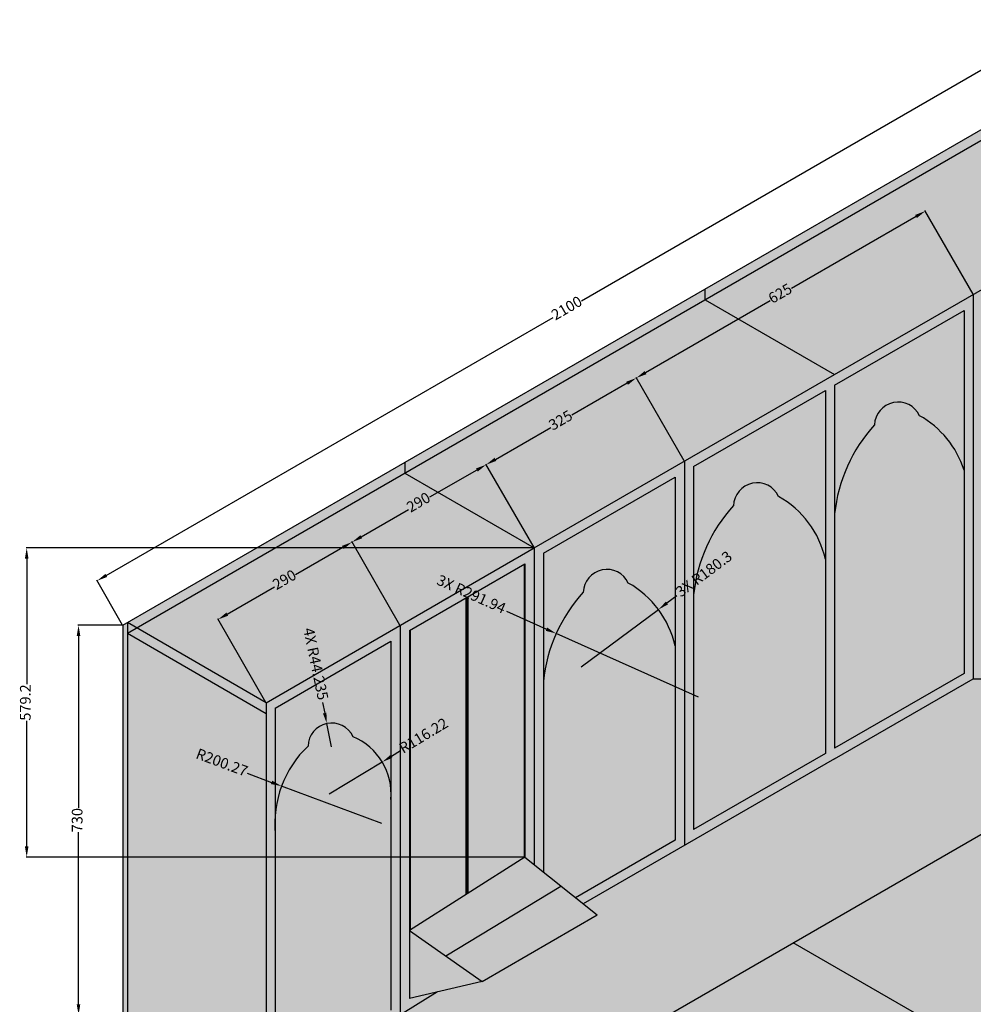
# Model space of a CAD drawing. Units: millimetres. Extents: x 78378 to 86415, y 148682 to 152721.
# Tile 12 of 18: x 78378 to 80164, y 150495 to 152340. Entities that reach past the tile are written whole.
import ezdxf

# ---------------------------------------------------------------- set-up
doc = ezdxf.new("R2010")
doc.units = ezdxf.units.MM
for name, color, linetype, lineweight in [('A-ANNO-DIMS', 2, 'Continuous', 18), ('A-ANNO-NPLT', 8, 'Continuous', 13), ('A-FURN', 4, 'Continuous', 25), ('A-FURN-PATT', 32, 'Continuous', 13)]:
    doc.layers.add(name, color=color, linetype=linetype, lineweight=lineweight)
doc.styles.get("Standard").update_dxf_attribs({"font": 'arial.ttf'})
doc.dimstyles.new('ISO-25', dxfattribs={"dimtxt": 20, "dimasz": 20, "dimexe": 1.25, "dimexo": 0.625, "dimtad": 0, "dimdec": 1, "dimtxsty": 'Standard', "dimcen": 2.5, "dimadec": 0, "dimazin": 0, "dimtfac": 1, "dimtdec": 1, "dimtmove": 0, "dimatfit": 3, "dimfxl": 1, "dimarcsym": 0})

# ---------------------------------------------------------------- blocks, each defined once
blk = doc.blocks.new('*D2')
at = {"layer": 'A-ANNO-DIMS', "color": 0, "lineweight": -2, "transparency": 16777216}
for p, q in [((80389.2, 152255.5), (80340.7, 152339.5)), ((80324, 152328.4), (79430.3, 151812.5)), ((78540, 151298.4), (79377.3, 151781.8)), ((78570.5, 151205.5), (78522.1, 151289.5))]:
    blk.add_line(p, q, dxfattribs=at)
at = {"layer": 'A-ANNO-DIMS', "color": 0, "transparency": 16777216}
for points in [[(80322.4, 152331.3), (80325.7, 152325.6), (80341.3, 152338.4)], [(78538.3, 151301.3), (78541.7, 151295.6), (78522.7, 151288.4)]]:
    blk.add_solid(points, dxfattribs=at)
at = {"layer": 'Defpoints', "color": 0, "transparency": 16777216}
for p in [(80341.3, 152338.4), (80389.5, 152255), (78570.9, 151205)]:
    blk.add_point(p, dxfattribs=at)
at = {"layer": 'A-ANNO-DIMS', "color": 0, "transparency": 16777216, "insert": (79403.8, 151797.2), "char_height": 20, "attachment_point": 5, "rotation": 30}
blk.add_mtext('2100', dxfattribs=at)
blk = doc.blocks.new('*D4')
at = {"layer": 'A-ANNO-DIMS', "color": 0, "lineweight": -2, "transparency": 16777216}
for p, q in [((78570.2, 151205), (78486.7, 151205)), ((78488, 151185), (78488, 150862.6)), ((78488, 150495), (78488, 150817.4)), ((78570.2, 150475), (78486.7, 150475))]:
    blk.add_line(p, q, dxfattribs=at)
at = {"layer": 'A-ANNO-DIMS', "color": 0, "transparency": 16777216}
for points in [[(78484.6, 151185), (78491.3, 151185), (78488, 151205)], [(78484.6, 150495), (78491.3, 150495), (78488, 150475)]]:
    blk.add_solid(points, dxfattribs=at)
at = {"layer": 'Defpoints', "color": 0, "transparency": 16777216}
for p in [(78570.9, 151205), (78488, 150475), (78570.9, 150475)]:
    blk.add_point(p, dxfattribs=at)
at = {"layer": 'A-ANNO-DIMS', "color": 0, "transparency": 16777216, "insert": (78488, 150840), "char_height": 20, "attachment_point": 5, "rotation": 90}
blk.add_mtext('730', dxfattribs=at)
blk = doc.blocks.new('*D14')
at = {"layer": 'A-ANNO-DIMS', "color": 0, "lineweight": -2, "transparency": 16777216}
for p, q in [((79090.2, 151205.5), (78999.8, 151362)), ((78983.2, 151350.9), (78894.7, 151299.8)), ((78766.6, 151225.9), (78855.1, 151277)), ((78839, 151060.5), (78748.7, 151217))]:
    blk.add_line(p, q, dxfattribs=at)
at = {"layer": 'A-ANNO-DIMS', "color": 0, "transparency": 16777216}
for points in [[(78981.5, 151353.8), (78984.8, 151348), (79000.5, 151360.9)], [(78765, 151228.8), (78768.3, 151223), (78749.3, 151215.9)]]:
    blk.add_solid(points, dxfattribs=at)
at = {"layer": 'Defpoints', "color": 0, "transparency": 16777216}
for p in [(79000.5, 151360.9), (79090.5, 151205), (78839.3, 151060)]:
    blk.add_point(p, dxfattribs=at)
at = {"layer": 'A-ANNO-DIMS', "color": 0, "transparency": 16777216, "insert": (78874.9, 151288.4), "char_height": 20, "attachment_point": 5, "rotation": 30}
blk.add_mtext('290', dxfattribs=at)
blk = doc.blocks.new('*D15')
at = {"layer": 'A-ANNO-DIMS', "color": 0, "lineweight": -2, "transparency": 16777216}
for p, q in [((79234.3, 151495.9), (79145.8, 151444.8)), ((79341.3, 151350.5), (79251, 151507)), ((79017.8, 151370.9), (79106.3, 151422)), ((79090.2, 151205.5), (78999.8, 151362))]:
    blk.add_line(p, q, dxfattribs=at)
at = {"layer": 'A-ANNO-DIMS', "color": 0, "transparency": 16777216}
for points in [[(79232.6, 151498.8), (79236, 151493), (79251.6, 151505.9)], [(79016.1, 151373.8), (79019.5, 151368), (79000.5, 151360.9)]]:
    blk.add_solid(points, dxfattribs=at)
at = {"layer": 'Defpoints', "color": 0, "transparency": 16777216}
for p in [(79251.6, 151505.9), (79341.6, 151350), (79090.5, 151205)]:
    blk.add_point(p, dxfattribs=at)
at = {"layer": 'A-ANNO-DIMS', "color": 0, "transparency": 16777216, "insert": (79126, 151433.4), "char_height": 20, "attachment_point": 5, "rotation": 30}
blk.add_mtext('290', dxfattribs=at)
blk = doc.blocks.new('*D16')
at = {"layer": 'A-ANNO-DIMS', "color": 0, "lineweight": -2, "transparency": 16777216}
for p, q in [((79515.8, 151658.4), (79412.1, 151598.5)), ((79622.8, 151513), (79532.5, 151669.5)), ((79268.9, 151515.9), (79372.6, 151575.7)), ((79341.3, 151350.5), (79251, 151507))]:
    blk.add_line(p, q, dxfattribs=at)
at = {"layer": 'A-ANNO-DIMS', "color": 0, "transparency": 16777216}
for points in [[(79514.1, 151661.3), (79517.4, 151655.5), (79533.1, 151668.4)], [(79267.3, 151518.8), (79270.6, 151513), (79251.6, 151505.9)]]:
    blk.add_solid(points, dxfattribs=at)
at = {"layer": 'Defpoints', "color": 0, "transparency": 16777216}
for p in [(79533.1, 151668.4), (79623.1, 151512.5), (79341.6, 151350)]:
    blk.add_point(p, dxfattribs=at)
at = {"layer": 'A-ANNO-DIMS', "color": 0, "transparency": 16777216, "insert": (79392.4, 151587.1), "char_height": 20, "attachment_point": 5, "rotation": 30}
blk.add_mtext('325', dxfattribs=at)
blk = doc.blocks.new('*D17')
at = {"layer": 'A-ANNO-DIMS', "color": 0, "lineweight": -2, "transparency": 16777216}
for p, q in [((80057, 151970.9), (79823.5, 151836.1)), ((80164, 151825.5), (80073.7, 151982)), ((79550.4, 151678.4), (79783.9, 151813.2)), ((79622.8, 151513), (79532.5, 151669.5))]:
    blk.add_line(p, q, dxfattribs=at)
at = {"layer": 'A-ANNO-DIMS', "color": 0, "transparency": 16777216}
for points in [[(80055.4, 151973.8), (80058.7, 151968), (80074.3, 151980.9)], [(79548.7, 151681.3), (79552.1, 151675.5), (79533.1, 151668.4)]]:
    blk.add_solid(points, dxfattribs=at)
at = {"layer": 'Defpoints', "color": 0, "transparency": 16777216}
for p in [(80074.3, 151980.9), (80164.3, 151825), (79623.1, 151512.5)]:
    blk.add_point(p, dxfattribs=at)
at = {"layer": 'A-ANNO-DIMS', "color": 0, "transparency": 16777216, "insert": (79803.7, 151824.6), "char_height": 20, "attachment_point": 5, "rotation": 30}
blk.add_mtext('625', dxfattribs=at)
blk = doc.blocks.new('*D18')
at = {"layer": 'A-ANNO-DIMS', "color": 0, "lineweight": -2, "transparency": 16777216}
for p, q in [((79341, 151350), (78389.6, 151350)), ((78390.9, 151330), (78390.9, 151094.7)), ((78390.9, 150790.8), (78390.9, 151026.1)), ((79323.7, 150770.8), (78389.6, 150770.8))]:
    blk.add_line(p, q, dxfattribs=at)
at = {"layer": 'A-ANNO-DIMS', "color": 0, "transparency": 16777216}
for points in [[(78387.5, 151330), (78394.2, 151330), (78390.9, 151350)], [(78387.5, 150790.8), (78394.2, 150790.8), (78390.9, 150770.8)]]:
    blk.add_solid(points, dxfattribs=at)
at = {"layer": 'Defpoints', "color": 0, "transparency": 16777216}
for p in [(78390.9, 151350), (79341.6, 151350), (79324.3, 150770.8)]:
    blk.add_point(p, dxfattribs=at)
at = {"layer": 'A-ANNO-DIMS', "color": 0, "transparency": 16777216, "insert": (78390.9, 151060.4), "char_height": 20, "attachment_point": 5, "rotation": 90}
blk.add_mtext('579.2', dxfattribs=at)
blk = doc.blocks.new('*D54')
at = {"layer": 'A-ANNO-DIMS', "color": 0, "lineweight": -2, "transparency": 16777216}
for p, q in [((79289.8, 151231.2), (79364.6, 151197.7)), ((79649.4, 151070.3), (79382.9, 151189.6))]:
    blk.add_line(p, q, dxfattribs=at)
at = {"layer": 'A-ANNO-DIMS', "color": 0, "transparency": 16777216}
blk.add_solid([(79366, 151200.8), (79363.3, 151194.7), (79382.9, 151189.6)], dxfattribs=at)
at = {"layer": 'Defpoints', "color": 0, "transparency": 16777216}
for p in [(79382.9, 151189.6), (79649.4, 151070.3)]:
    blk.add_point(p, dxfattribs=at)
at = {"layer": 'A-ANNO-DIMS', "color": 0, "transparency": 16777216, "insert": (79223, 151261.1), "char_height": 20, "attachment_point": 5, "rotation": 335.8929}
blk.add_mtext('3X R291.94', dxfattribs=at)
blk = doc.blocks.new('*D55')
at = {"layer": 'A-ANNO-DIMS', "color": 0, "lineweight": -2, "transparency": 16777216}
for p, q in [((79608.7, 151260.2), (79590.4, 151246.6)), ((79429.9, 151126.9), (79574.4, 151234.7))]:
    blk.add_line(p, q, dxfattribs=at)
at = {"layer": 'A-ANNO-DIMS', "color": 0, "transparency": 16777216}
blk.add_solid([(79588.4, 151249.3), (79592.4, 151244), (79574.4, 151234.7)], dxfattribs=at)
at = {"layer": 'Defpoints', "color": 0, "transparency": 16777216}
for p in [(79574.4, 151234.7), (79429.9, 151126.9)]:
    blk.add_point(p, dxfattribs=at)
at = {"layer": 'A-ANNO-DIMS', "color": 0, "transparency": 16777216, "insert": (79661.1, 151299.3), "char_height": 20, "attachment_point": 5, "rotation": 36.7052}
blk.add_mtext('3X R180.3', dxfattribs=at)
blk = doc.blocks.new('*D56')
at = {"layer": 'A-ANNO-DIMS', "color": 0, "lineweight": -2, "transparency": 16777216}
for p, q in [((78945.1, 151060.1), (78949.2, 151040.5)), ((78962.2, 150977.6), (78953.2, 151020.9))]:
    blk.add_line(p, q, dxfattribs=at)
at = {"layer": 'A-ANNO-DIMS', "color": 0, "transparency": 16777216}
blk.add_solid([(78952.4, 151041.2), (78945.9, 151039.9), (78953.2, 151020.9)], dxfattribs=at)
at = {"layer": 'Defpoints', "color": 0, "transparency": 16777216}
for p in [(78953.2, 151020.9), (78962.2, 150977.6)]:
    blk.add_point(p, dxfattribs=at)
at = {"layer": 'A-ANNO-DIMS', "color": 0, "transparency": 16777216, "insert": (78930.2, 151132.3), "char_height": 20, "attachment_point": 5, "rotation": 281.693}
blk.add_mtext('4X R44.235', dxfattribs=at)
blk = doc.blocks.new('*D57')
at = {"layer": 'A-ANNO-DIMS', "color": 0, "lineweight": -2, "transparency": 16777216}
for p, q in [((78804.2, 150927.7), (78849.6, 150910.8)), ((79056, 150833.8), (78868.4, 150903.8))]:
    blk.add_line(p, q, dxfattribs=at)
at = {"layer": 'A-ANNO-DIMS', "color": 0, "transparency": 16777216}
blk.add_solid([(78850.8, 150913.9), (78848.4, 150907.6), (78868.4, 150903.8)], dxfattribs=at)
at = {"layer": 'Defpoints', "color": 0, "transparency": 16777216}
for p in [(78868.4, 150903.8), (79056, 150833.8)]:
    blk.add_point(p, dxfattribs=at)
at = {"layer": 'A-ANNO-DIMS', "color": 0, "transparency": 16777216, "insert": (78755.8, 150945.8), "char_height": 20, "attachment_point": 5, "rotation": 339.5422}
blk.add_mtext('R200.27', dxfattribs=at)
blk = doc.blocks.new('*D58')
at = {"layer": 'A-ANNO-DIMS', "color": 0, "lineweight": -2, "transparency": 16777216}
for p, q in [((79091.3, 150969.7), (79074.1, 150959.4)), ((78957.4, 150889.1), (79057, 150949))]:
    blk.add_line(p, q, dxfattribs=at)
at = {"layer": 'A-ANNO-DIMS', "color": 0, "transparency": 16777216}
blk.add_solid([(79072.4, 150962.2), (79075.8, 150956.5), (79057, 150949)], dxfattribs=at)
at = {"layer": 'Defpoints', "color": 0, "transparency": 16777216}
for p in [(79057, 150949), (78957.4, 150889.1)]:
    blk.add_point(p, dxfattribs=at)
at = {"layer": 'A-ANNO-DIMS', "color": 0, "transparency": 16777216, "insert": (79135.5, 150996.3), "char_height": 20, "attachment_point": 5, "rotation": 31.0485}
blk.add_mtext('R116.22', dxfattribs=at)

msp = doc.modelspace()

# ---------------------------------------------------------------- hatches: boundary and pattern name
at = {"layer": 'A-FURN-PATT'}
h = msp.add_hatch(color=256, dxfattribs=at)
h.dxf.hatch_style = 1
h.paths.add_polyline_path([(80389.5131, 152235.0076), (80389.5131, 152255.0076), (79662.0518, 151835.0076), (79662.0518, 151815.0076)])
h.paths.add_polyline_path([(79662.0518, 151815.0076), (79662.0518, 151835.0076), (79099.1352, 151510.0076), (79099.1352, 151490.0076)])
h.paths.add_polyline_path([(79099.1352, 151490.0076), (79099.1352, 151510.0076), (78579.52, 151210.0076), (78596.8405, 151200.0076)])
h.paths.add_polyline_path([(80632.0002, 152115.0076), (80632.0002, 152095.0076), (80867.7794, 151958.8805), (80867.7794, 151978.8805)])
h.paths.add_polyline_path([(80389.5131, 152255.0076), (80389.5131, 152235.0076), (80632.0002, 152095.0076), (80632.0002, 152115.0076)])
h = msp.add_hatch(color=256, dxfattribs=at)
h.dxf.hatch_style = 1
h.paths.add_polyline_path([(78839.3276, 151040.0076), (78579.52, 151190.0076), (78579.52, 150470.0076), (78839.3276, 150320.0076)])
h.paths.add_polyline_path([(79073.1545, 150899.6469, 0.277779695), (79002.2645, 150996.3205, 0.791083931), (78917.9567, 150978.8719, 0.180448316), (78856.6481, 150853.0138), (78856.6481, 150350.6973), (79073.1545, 150484.318)])
h.paths.add_polyline_path([(79073.1545, 151175.0076), (78856.6481, 151050.0076), (78856.6481, 150853.0138, -0.180448316), (78917.9567, 150978.8719, -0.791083931), (79002.2645, 150996.3205, -0.277779695), (79073.1545, 150899.6469)])
h.paths.add_polyline_path([(79341.6224, 151350.0076), (79099.1352, 151490.0076), (78596.8405, 151200.0076), (78839.3276, 151060.0076)])
h.paths.add_polyline_path([(79904.5389, 151675.0076), (79662.0518, 151815.0076), (79099.1352, 151490.0076), (79341.6224, 151350.0076)])
h.paths.add_polyline_path([(80389.5131, 151955.0076), (80389.5131, 152235.0076), (79662.0518, 151815.0076), (79904.5389, 151675.0076)])
h.paths.add_polyline_path([(80389.5131, 151955.0076), (80164.3465, 151825.0076), (80164.3465, 151105.0076), (80614.6797, 151105.0076), (80614.6797, 151825.0076)])
edge = h.paths.add_edge_path(flags=16)
edge.add_spline(control_points=[(80216.308, 151728.251), (80227.1854, 151732.981), (80256.3301, 151745.6544), (80298.41, 151761.9595), (80340.2597, 151805.855), (80391.0771, 151782.0404), (80454.0396, 151805.7581), (80496.5007, 151742.4095), (80543.8218, 151733.4043), (80562.7182, 151729.8083)], knot_values=[0, 0, 0, 0, 35.543746761, 95.235753469, 136.367675126, 200.932981967, 236.726410811, 322.889934976, 380.170273667, 380.170273667, 380.170273667, 380.170273667], degree=3, periodic=0)
edge.add_line((80562.7182, 151729.8083), (80562.7182, 151165.0076))
edge.add_line((80562.7182, 151165.0076), (80216.308, 151165.0076))
edge.add_line((80216.308, 151165.0076), (80216.308, 151728.251))
h.paths.add_polyline_path([(80632.0002, 152095.0076), (80389.5131, 152235.0076), (80389.5131, 151955.0076), (80614.6797, 151825.0076), (80632.0002, 151815.0076)])
h.paths.add_polyline_path([(80867.7794, 151958.8805), (80632.0002, 152095.0076), (80632.0002, 151815.0076), (80632.0002, 151510.0076), (80867.7794, 151373.8805)])
h.paths.add_polyline_path([(80147.026, 151495.8203, 0.18918979), (80063.5671, 151597.7244, 0.788261355), (79979.2691, 151580.5832, 0.160726132), (79904.5389, 151413.5769), (79904.5389, 150955.0076), (80147.026, 151095.0076)])
h.paths.add_polyline_path([(80147.026, 151815.0076), (79904.5389, 151675.0076), (79904.5389, 151413.5769, -0.160726132), (79979.2691, 151580.5832, -0.788261355), (80063.5671, 151597.7244, -0.18918979), (80147.026, 151495.8203)])
h.paths.add_polyline_path([(79887.2184, 151645.0076), (79640.4011, 151502.5076), (79640.4011, 151262.3325, -0.160726132), (79715.1313, 151429.3387, -0.788261355), (79799.4294, 151446.48, -0.21290578), (79887.2184, 151328.7247)])
h.paths.add_polyline_path([(79799.4294, 151446.48, 0.788261355), (79715.1313, 151429.3387, 0.160726132), (79640.4011, 151262.3325), (79640.4011, 150822.5076), (79887.2184, 150965.0076), (79887.2184, 151328.7247, 0.21290578)])
h.paths.add_polyline_path([(79605.7601, 151482.5076), (79358.9429, 151340.0076), (79358.9429, 151100.0701, -0.160726132), (79433.6731, 151267.0764, -0.788261355), (79517.9711, 151284.2176, -0.21290578), (79605.7601, 151166.4623)])
h.paths.add_polyline_path([(79605.7601, 151166.4623, 0.21290578), (79517.9711, 151284.2176, 0.788261355), (79433.6731, 151267.0764, 0.160726132), (79358.9429, 151100.0701), (79358.9429, 150742.9831), (79419.0877, 150694.7323), (79605.7601, 150802.5076)])
edge = h.paths.add_edge_path(flags=0)
edge.add_spline(control_points=[(81152.4356, 151098.7676), (81105.7208, 151145.9466), (81038.6136, 151213.7208), (80882.3866, 151214.1938), (80797.4434, 151311.2997), (80711.8686, 151340.3754), (80681.7691, 151350.6023)], knot_values=[0, 0, 0, 0, 188.233441, 270.4032752, 445.451792012, 540.428588287, 540.428588287, 540.428588287, 540.428588287], degree=3, periodic=0)
edge.add_line((80683.4538, 151350.0269), (80683.4538, 151104.8792))
edge.add_line((80683.4538, 151104.8792), (81152.4356, 150851.399))
edge.add_line((81152.4356, 150851.399), (81152.4356, 151098.7676))
edge = h.paths.add_edge_path(flags=0)
edge.add_spline(control_points=[(80912.9018, 151027.1103), (80892.3742, 151034.1027), (80860.1663, 151045.0739), (80835.5097, 151068.1214), (80826.5679, 151076.4797)], knot_values=[0, 0, 0, 0, 63.98405104, 100.391424282, 100.391424282, 100.391424282, 100.391424282], degree=3, periodic=0)
edge.add_arc((80830.0414, 151081.2992), 5.9407, 100.9277276, 234.2187381, ccw=False)
edge.add_spline(control_points=[(80828.9152, 151087.1322), (80837.857, 151078.7739), (80862.5136, 151055.7263), (80894.7215, 151044.7552), (80915.2491, 151037.7628)], knot_values=[0, 0, 0, 0, 36.407373242, 100.391424282, 100.391424282, 100.391424282, 100.391424282], degree=3, periodic=0)
edge.add_arc((80914.7882, 151032.2795), 5.5026, -107.9540399, 85.195579, ccw=False)
h.paths.add_polyline_path([(81238.218, 151110.0076), (80632.0002, 151460.0076), (80632.0002, 151105.0076), (81238.218, 150755.0076)])
edge = h.paths.add_edge_path(flags=16)
edge.add_line((81152.4356, 150851.399), (80683.4538, 151104.8792))
edge.add_line((80683.4538, 151104.8792), (80683.4538, 151350.0279))
edge.add_spline(control_points=[(80681.7691, 151350.6023), (80711.8686, 151340.3754), (80797.4434, 151311.2997), (80882.3866, 151214.1938), (81038.6136, 151213.7208), (81105.7208, 151145.9466), (81152.4356, 151098.7676)], knot_values=[0, 0, 0, 0, 94.976796275, 270.025313088, 352.195147288, 540.428588287, 540.428588287, 540.428588287, 540.428588287], degree=3, periodic=0)
edge.add_line((81152.4356, 151098.7676), (81152.4356, 150851.399))
edge = h.paths.add_edge_path(flags=0)
edge.add_spline(control_points=[(80912.9018, 151027.1103), (80892.3742, 151034.1027), (80860.1663, 151045.0739), (80835.5097, 151068.1214), (80826.5679, 151076.4797)], knot_values=[0, 0, 0, 0, 63.98405104, 100.391424282, 100.391424282, 100.391424282, 100.391424282], degree=3, periodic=0)
edge.add_arc((80830.0414, 151081.2992), 5.9407, 100.9277276, 234.2187381, ccw=False)
edge.add_spline(control_points=[(80828.9152, 151087.1322), (80837.857, 151078.7739), (80862.5136, 151055.7263), (80894.7215, 151044.7552), (80915.2491, 151037.7628)], knot_values=[0, 0, 0, 0, 36.407373242, 100.391424282, 100.391424282, 100.391424282, 100.391424282], degree=3, periodic=0)
edge.add_arc((80914.7882, 151032.2795), 5.5026, -107.7417882, 85.195579, ccw=False)
h.paths.add_polyline_path([(81498.0256, 151255.0076), (81238.218, 151110.0076), (81238.218, 150755.0076), (81498.0256, 150905.0076)])
edge = h.paths.add_edge_path(flags=16)
edge.add_spline(control_points=[(81152.4356, 151098.7676), (81105.7208, 151145.9466), (81038.6136, 151213.7208), (80882.3866, 151214.1938), (80797.4434, 151311.2997), (80711.8686, 151340.3754), (80681.7691, 151350.6023)], knot_values=[0, 0, 0, 0, 188.233441, 270.4032752, 445.451792012, 540.428588287, 540.428588287, 540.428588287, 540.428588287], degree=3, periodic=0)
edge.add_line((80683.4538, 151350.0279), (80683.4538, 151104.8792))
edge.add_line((80683.4538, 151104.8792), (81152.4356, 150851.399))
edge.add_line((81152.4356, 150851.399), (81152.4356, 151098.7676))
h.paths.add_polyline_path([(81453.9904, 151280.4314), (80867.7794, 151618.8805), (80867.7794, 151373.8805), (81238.218, 151160.0076)])
edge = h.paths.add_edge_path(flags=16)
edge.add_line((81189.2304, 151297.6373), (81114.4166, 151300.2154))
edge.add_arc((81412.0967, 151394.0167), 312.1092, 179.7569303, 197.4900342, ccw=False)
edge.add_ellipse((81154.0183, 151392.0436), major_axis=(-54.0264, 3.6301), ratio=0.221796934, start_angle=0, end_angle=0.3517985, ccw=False)
edge.add_ellipse((81154.0183, 151392.0436), major_axis=(-54.0264, 3.6301), ratio=0.221796934, start_angle=180, end_angle=360, ccw=False)
edge.add_spline(control_points=[(81196.1844, 151321.9476), (81224.9802, 151347.1455), (81266.8846, 151383.8144), (81222.0354, 151387.0304), (81208.0056, 151388.0364)], knot_values=[0, 0, 0, 0, 75.091751734, 109.275804387, 109.275804387, 109.275804387, 109.275804387], degree=3, periodic=0)
edge.add_arc((80751.9112, 151435.6145), 458.5693, 342.4891602, 345.646172, ccw=False)
edge = h.paths.add_edge_path(flags=0)
edge.add_spline(control_points=[(81196.6193, 151323.657), (81197.893, 151324.7717), (81199.1654, 151325.8858), (81209.0233, 151334.5343), (81217.3959, 151341.9835), (81228.0928, 151352.5012), (81231.3883, 151355.9524), (81236.9493, 151362.4395), (81239.214, 151365.4773), (81241.4987, 151369.416), (81242.064, 151370.5542), (81242.9187, 151372.6971), (81243.2076, 151373.7015), (81243.5012, 151375.5539), (81243.5065, 151376.4), (81243.2432, 151377.9407), (81242.9775, 151378.6373), (81242.1402, 151379.937), (81241.5659, 151380.5416), (81240.2039, 151381.533), (81239.4963, 151381.9384), (81237.0619, 151383.0663), (81235.0242, 151383.6999), (81230.352, 151384.7569), (81227.7173, 151385.1826), (81221.9118, 151385.9145), (81218.7193, 151386.2133), (81213.7912, 151386.6115), (81212.1252, 151386.7359), (81209.6196, 151386.9181), (81208.7865, 151386.9779), (81207.9009, 151387.0432)], knot_values=[0.015487437, 0.015487437, 0.015487437, 0.015487437, 3.337879569, 3.337879569, 25.851306242, 25.851306242, 37.52811308, 37.52811308, 49.204919918, 49.204919918, 54.285093801, 54.285093801, 59.365267683, 59.365267683, 64.445441566, 64.445441566, 69.525615449, 69.525615449, 74.605789331, 74.605789331, 78.493667847, 78.493667847, 86.255670953, 86.255670953, 94.017674059, 94.017674059, 102.202265559, 102.202265559, 106.294561309, 106.294561309, 108.325221747, 108.325221747, 108.325221747, 108.325221747], degree=3, periodic=0)
edge = h.paths.add_edge_path(flags=16)
edge.add_arc((81034.1732, 151350.4693), 42.5822, 231.2679035, 306.151846, ccw=False)
edge.add_line((81007.5303, 151317.2517), (81007.5303, 151395.181))
edge.add_ellipse((81033.412, 151394.7791), major_axis=(-25.8816, 0.4538), ratio=0.23894509, start_angle=0, end_angle=0.1147075, ccw=False)
edge.add_ellipse((81033.412, 151394.7791), major_axis=(-25.8816, 0.4538), ratio=0.23894509, start_angle=181.1677709, end_angle=358.9476457, ccw=False)
edge.add_ellipse((81033.412, 151395.7791), major_axis=(-25.8816, 0.4538), ratio=0.23894509, start_angle=180, end_angle=360.1147075, ccw=False)
edge.add_ellipse((81033.412, 151395.7791), major_axis=(-25.8816, 0.4538), ratio=0.23894509, start_angle=178.9476457, end_angle=180, ccw=False)
edge.add_line((81059.2936, 151395.1778), (81059.2936, 151394.3772))
edge.add_ellipse((81033.412, 151394.7791), major_axis=(-25.8816, 0.4538), ratio=0.23894509, start_angle=180, end_angle=180.1147075, ccw=False)
edge.add_ellipse((81033.412, 151394.7791), major_axis=(-25.8816, 0.4538), ratio=0.23894509, start_angle=3.6903098, end_angle=176.4406503, ccw=False)
edge.add_line((81059.2936, 151393.3388), (81059.2936, 151316.086))
h.paths.add_polyline_path([(80951.9355, 151343.9568), (80909.6838, 151362.4635), (80904.0219, 151443.9615, -0.381333076), (80987.2169, 151411.3717)], flags=16)
h = msp.add_hatch(color=256, dxfattribs=at)
h.dxf.hatch_style = 1
h.paths.add_polyline_path([(80389.8136, 150935.1811), (80389.5131, 151105.0076), (80164.3465, 151105.0076), (79904.5389, 150955.0076), (79433.5848, 150683.1022), (79459.4128, 150662.3818), (79243.9048, 150537.9582), (79160.4069, 150518.1674), (78839.3276, 150320.0076), (78579.52, 150470.0076), (78570.8597, 150475.0076), (78570.8597, 150465.0076), (78570.8597, 149885.0076)])
h.paths.add_polyline_path([(80086.4042, 150460.0076), (79826.5966, 150610.0076), (78570.8597, 149885.0076), (78830.6674, 149735.0076)])
h.paths.add_polyline_path([(79540.8001, 150161.0557), (79217.3967, 149974.3386), (78980.9166, 150110.8705), (79304.32, 150297.5875)], flags=16)
h.paths.add_polyline_path([(79506.159, 150161.0557), (79217.3967, 149994.3386), (79015.5576, 150110.8705), (79304.32, 150277.5875)], flags=0)
edge = h.paths.add_edge_path(flags=0)
edge.add_arc((79247.8636, 150177.1541), 137.9799, 256.0025928, 293.5594109)
edge.add_arc((79240.7671, 150078.2605), 68.0855, 336.099104, 387.3696877)
edge.add_ellipse((79258.3074, 150109.4852), major_axis=(-42.6234, -1.6591), ratio=0.160428429, start_angle=0, end_angle=179.0977279, ccw=False)
edge.add_arc((79285.2112, 150074.2509), 77.2096, 155.1233104, 203.6557939)
edge = h.paths.add_edge_path(flags=0)
edge.add_ellipse((79258.6958, 150110.8297), major_axis=(-42.6234, -1.6591), ratio=0.160428429, start_angle=350.6039412, end_angle=356.2289762)
edge.add_line((79219.169, 150111.8937), (79218.3268, 150109.4141))
edge.add_arc((79262.4675, 150032.9602), 88.2813, 112.3931229, 120, ccw=False)
h.paths.add_polyline_path([(79287.0625, 150086.9703, -0.247702064), (79288.1967, 150077.2955, -0.390476513), (79265.4731, 150072.5438, -0.487261526), (79264.079, 150082.3769, 0.395604326)], flags=0)
h.paths.add_polyline_path([(80389.5131, 150935.0076), (79826.5966, 150610.0076), (80086.4042, 150460.0076), (80692.622, 150460.0076), (80952.4296, 150610.0076)])
edge = h.paths.add_edge_path(flags=16)
edge.add_ellipse((80392.4466, 150825.601), major_axis=(-133.0757, 7.722), ratio=0.42449957, start_angle=0, end_angle=360)
edge = h.paths.add_edge_path(flags=0)
edge.add_spline(control_points=[(80269.3541, 150832.7436), (80269.2919, 150831.672), (80269.3503, 150830.5922), (80269.7341, 150828.3361), (80270.0612, 150827.1587), (80271.0461, 150824.6748), (80271.7052, 150823.3692), (80273.4061, 150820.6503), (80274.4481, 150819.2381), (80276.9366, 150816.3509), (80278.3828, 150814.8762), (80282.5858, 150811.0913), (80285.6261, 150808.7701), (80292.6031, 150804.2267), (80296.5388, 150802.0041), (80305.195, 150797.7581), (80309.9151, 150795.7344), (80320.0112, 150791.96), (80325.387, 150790.2092), (80339.2162, 150786.315), (80347.9578, 150784.3563), (80366.0679, 150781.2568), (80375.4359, 150780.1158), (80394.3093, 150778.7158), (80403.8142, 150778.4568), (80422.4656, 150778.8319), (80431.6115, 150779.4662), (80449.0608, 150781.5838), (80457.3636, 150783.0675), (80472.6699, 150786.7766), (80479.6726, 150789.0033), (80490.1894, 150793.2813), (80494.1268, 150795.1967), (80501.0146, 150799.1885), (80503.9632, 150801.2651), (80508.2066, 150804.9015), (80509.73, 150806.4609), (80512.1996, 150809.4942), (80513.1456, 150810.9657), (80514.4291, 150813.5431), (80514.8436, 150814.6688), (80515.3984, 150816.8625), (80515.5405, 150817.9315), (80515.5801, 150820.098), (80515.4773, 150821.1978), (80514.9905, 150823.5062), (80514.6047, 150824.7154), (80513.4854, 150827.2641), (80512.7511, 150828.6027), (80510.8872, 150831.3809), (80509.7578, 150832.8196), (80507.0873, 150835.7513), (80505.5466, 150837.2439), (80501.0624, 150841.0944), (80497.8199, 150843.4576), (80490.4174, 150848.062), (80486.2582, 150850.3037), (80477.1448, 150854.5643), (80472.1909, 150856.5835), (80461.6275, 150860.3245), (80456.0182, 150862.0465), (80441.7332, 150865.8127), (80432.7885, 150867.6675), (80414.3391, 150870.5317), (80404.8349, 150871.5411), (80385.7707, 150872.6572), (80376.2113, 150872.764), (80357.5444, 150872.0728), (80348.4375, 150871.2748), (80331.1682, 150868.83), (80323.0064, 150867.1827), (80309.472, 150863.5363), (80303.8628, 150861.6593), (80293.8018, 150857.5401), (80289.3512, 150855.2969), (80282.7757, 150851.2345), (80280.3473, 150849.4579), (80276.2606, 150845.9127), (80274.604, 150844.1458), (80272.3157, 150841.1243), (80271.5358, 150839.8454), (80270.3496, 150837.3879), (80269.9417, 150836.2101), (80269.5065, 150834.2815), (80269.3988, 150833.5143), (80269.3541, 150832.7436)], knot_values=[0, 0, 0, 0, 0.09750046, 0.09750046, 0.19500092, 0.19500092, 0.292501379, 0.292501379, 0.390001839, 0.390001839, 0.487502299, 0.487502299, 0.638803224, 0.638803224, 0.790104149, 0.790104149, 0.941405074, 0.941405074, 1.092705999, 1.092705999, 1.312817101, 1.312817101, 1.532928203, 1.532928203, 1.753039304, 1.753039304, 1.973150406, 1.973150406, 2.193261508, 2.193261508, 2.413372609, 2.413372609, 2.569860633, 2.569860633, 2.726348657, 2.726348657, 2.844186582, 2.844186582, 2.962024507, 2.962024507, 3.060233876, 3.060233876, 3.158443245, 3.158443245, 3.256652615, 3.256652615, 3.354861984, 3.354861984, 3.453071354, 3.453071354, 3.551280723, 3.551280723, 3.649490093, 3.649490093, 3.80392773, 3.80392773, 3.958365368, 3.958365368, 4.112803006, 4.112803006, 4.267240644, 4.267240644, 4.489203495, 4.489203495, 4.711166346, 4.711166346, 4.933129197, 4.933129197, 5.155092048, 5.155092048, 5.3770549, 5.3770549, 5.557853609, 5.557853609, 5.738652318, 5.738652318, 5.872395556, 5.872395556, 6.006138794, 6.006138794, 6.109604996, 6.109604996, 6.213071198, 6.213071198, 6.283185307, 6.283185307, 6.283185307, 6.283185307], degree=3, periodic=0)
edge = h.paths.add_edge_path(flags=0)
edge.add_ellipse((80392.4466, 150825.601), major_axis=(-101.8398, 3.3923), ratio=0.403492477, start_angle=0, end_angle=360)
edge = h.paths.add_edge_path(flags=0)
edge.add_ellipse((80391.1657, 150858.3746), major_axis=(9.0882, -0.6733), ratio=0.351354129, start_angle=0, end_angle=360)
h.paths.add_polyline_path([(80952.4296, 150610.0076), (80692.622, 150460.0076), (81361.2342, 150073.9842), (81649.9628, 150052.7286), (81766.4935, 150120.0076), (81766.4935, 150140.0076), (81564.9025, 150256.3963), (81564.8884, 150096.1963), (81538.9076, 150111.1963), (81538.9217, 150271.3963)])
h.paths.add_polyline_path([(81539.0357, 151571.3305), (80867.7794, 151958.8805), (80867.7794, 151618.8805), (81498.0256, 151255.0076), (81498.0256, 150905.0076), (81238.218, 150755.0076), (81538.9488, 150581.3806)])
h.paths.add_polyline_path([(81766.4935, 151440.0076), (81565.0164, 151556.3305), (81564.9296, 150566.3806), (81766.4935, 150450.0076)])
edge = h.paths.add_edge_path()
edge.add_line((81564.9296, 150566.3806), (81564.9137, 150384.6289))
edge.add_ellipse((81552.1304, 150358.5718), major_axis=(52.6272, 3.506), ratio=0.495899055, start_angle=367.5169757, end_angle=420.0564686, ccw=False)
edge.add_ellipse((81552.1304, 150358.5718), major_axis=(52.6272, 3.506), ratio=0.495899055, start_angle=351.729742, end_angle=367.5169757, ccw=False)
edge.add_ellipse((81552.1304, 150345.5016), major_axis=(52.6272, 3.506), ratio=0.495899055, start_angle=352.5116949, end_angle=366.3006092, ccw=False)
edge.add_line((81603.4463, 150342.2039), (81603.5064, 150340.4475))
edge.add_ellipse((81552.1304, 150332.128), major_axis=(52.6272, 3.506), ratio=0.495899055, start_angle=353.6729654, end_angle=365.3867997, ccw=False)
edge.add_ellipse((81552.1304, 150332.128), major_axis=(52.6272, 3.506), ratio=0.495899055, start_angle=350.9388331, end_angle=353.6729654)
edge.add_line((81603.8688, 150329.855), (81604.0442, 150324.7302))
edge.add_ellipse((81552.1304, 150317.7418), major_axis=(52.6272, 3.506), ratio=0.495899055, start_angle=355.2176746, end_angle=363.8553364, ccw=False)
edge.add_ellipse((81552.1304, 150317.7418), major_axis=(52.6272, 3.506), ratio=0.495899055, start_angle=341.3250873, end_angle=355.2176746, ccw=False)
edge.add_ellipse((81552.1304, 150317.7418), major_axis=(52.6272, 3.506), ratio=0.495899055, start_angle=293.4661701, end_angle=341.3250873, ccw=False)
edge.add_line((81564.9057, 150292.9664), (81564.9025, 150256.3963))
edge.add_line((81564.9025, 150256.3963), (81766.4935, 150140.0076))
edge.add_line((81766.4935, 150140.0076), (81766.4935, 150450.0076))
edge.add_line((81766.4935, 150450.0076), (81564.9296, 150566.3806))
h.paths.add_polyline_path([(81525.5713, 150321.598), (81526.5985, 150321.3069), (81528.6771, 150320.947)])
h.paths.add_polyline_path([(81512.7903, 150326.1129), (81514.5058, 150325.3887), (81512.538, 150326.2678)])
h.paths.add_polyline_path([(81533.2148, 150320.1615), (81534.6952, 150319.9052), (81536.5995, 150319.7557)])
h.paths.add_polyline_path([(81518.622, 150323.6513), (81519.227, 150323.3959), (81521.289, 150322.8116)])
h.paths.add_polyline_path([(81501.2183, 150336.2599), (81500.3543, 150338.1339), (81499.7815, 150340.0494), (81499.5032, 150341.9955), (81499.5032, 150343.7257), (81499.7584, 150345.5905), (81500.2766, 150347.4549), (81501.0551, 150349.3095), (81501.0967, 150349.3937), (81501.1389, 150349.4778), (81500.9978, 150349.7496), (81500.8628, 150350.0225), (81499.5032, 150355.0658), (81499.9591, 150359.5002), (81501.8982, 150363.9083), (81505.2653, 150368.1646), (81509.9647, 150372.1482), (81515.8627, 150375.7459), (81522.7918, 150378.8553), (81530.555, 150381.3882), (81538.9315, 150383.2724), (81538.9488, 150581.3806), (80632.0002, 151105.0076), (80389.5131, 151105.0076), (80389.8142, 150934.8338), (80952.4296, 150610.0076), (81538.9217, 150271.3963), (81538.9234, 150291.7194), (81538.8752, 150291.721), (81530.1915, 150292.8239), (81522.1802, 150294.6904), (81515.0866, 150297.2633), (81509.8635, 150299.9959), (81505.6084, 150303.1351), (81502.419, 150306.6088), (81500.3683, 150310.3375), (81499.5032, 150314.2358), (81499.5032, 150315.9659), (81499.8206, 150318.1159), (81500.487, 150320.2634), (81501.4979, 150322.3941), (81500.487, 150324.4233), (81499.8206, 150326.5039), (81499.5032, 150328.622), (81499.5032, 150330.3521), (81499.7815, 150332.3262), (81500.3543, 150334.2992)])
h = msp.add_hatch(color=256, dxfattribs=at)
h.dxf.hatch_style = 1
h.paths.add_polyline_path([(79090.475, 151205.0076), (78839.3276, 151060.0076), (78839.3276, 150320.0076), (79090.475, 150475.0076)])
h.paths.add_polyline_path([(79073.1545, 151175.0076), (79073.1545, 150899.6469, -0.04544363), (79073.1545, 150878.5653), (79073.1545, 150484.318), (78856.6481, 150350.6973), (78856.6481, 150814.5249, -0.048157161), (78856.6481, 150853.0138), (78856.6481, 151050.0076)], flags=16)
h.paths.add_polyline_path([(79358.9429, 151340.0076), (79605.7601, 151482.5076), (79605.7601, 150802.5076), (79419.0877, 150694.7323), (79433.5848, 150683.1022), (79623.0806, 150792.5076), (79623.0806, 151512.5076), (79341.6224, 151350.0076), (79341.6224, 150756.8784), (79358.9429, 150742.9831)])
h.paths.add_polyline_path([(79341.6224, 151350.0076), (79090.475, 151205.0076), (79090.475, 150475.0076), (79160.4069, 150518.1674), (79107.7955, 150505.6973), (79107.7955, 151195.0076), (79109.5275, 151196.0076), (79324.3018, 151320.0076), (79324.3018, 150770.7736), (79341.6224, 150756.8784)])
h.paths.add_polyline_path([(79887.2184, 151645.0076), (79887.2184, 151665.0076), (79623.0806, 151512.5076), (79623.0806, 150792.5076), (79887.2184, 150945.0076), (79887.2184, 150965.0076), (79640.4011, 150822.5076), (79640.4011, 151502.5076)])
h.paths.add_polyline_path([(79904.5389, 151655.0076), (79887.2184, 151645.0076), (79887.2184, 150965.0076), (79904.5389, 150975.0076)])
h.paths.add_polyline_path([(80164.3465, 151825.0076), (80147.026, 151815.0076), (80147.026, 151095.0076), (80164.3465, 151105.0076)])
h.paths.add_polyline_path([(80632.0002, 151510.0076), (80632.0002, 151490.0076), (81238.218, 151140.0076), (81471.6045, 151270.2619), (81453.9904, 151280.4314), (81238.218, 151160.0076)])
h.paths.add_polyline_path([(80632.0002, 151490.0076), (80632.0002, 151470.0076), (81238.218, 151120.0076), (81489.2186, 151260.0924), (81471.6045, 151270.2619), (81238.218, 151140.0076)])
h.paths.add_polyline_path([(80632.0002, 151460.0076), (80632.0002, 151105.0076), (81238.218, 150755.0076), (81238.218, 151110.0076)])
edge = h.paths.add_edge_path(flags=16)
edge.add_spline(control_points=[(80681.7691, 151350.6023), (80711.8686, 151340.3754), (80797.4434, 151311.2997), (80882.3866, 151214.1938), (81038.6136, 151213.7208), (81105.7208, 151145.9466), (81152.4356, 151098.7676)], knot_values=[0, 0, 0, 0, 94.976796275, 270.025313088, 352.195147288, 540.428588287, 540.428588287, 540.428588287, 540.428588287], degree=3, periodic=0)
edge.add_line((81152.4356, 151098.7676), (81152.4356, 150851.399))
edge.add_line((81152.4356, 150851.399), (80683.4538, 151104.8792))
edge.add_line((80683.4538, 151104.8792), (80683.4538, 151350.027))
edge = h.paths.add_edge_path(flags=0)
edge.add_spline(control_points=[(80828.9152, 151087.1322), (80837.857, 151078.7739), (80862.5136, 151055.7263), (80894.7215, 151044.7552), (80915.2491, 151037.7628)], knot_values=[0, 0, 0, 0, 36.407373242, 100.391424282, 100.391424282, 100.391424282, 100.391424282], degree=3, periodic=0)
edge.add_arc((80914.7882, 151032.2795), 5.5026, -107.9540399, 85.195579, ccw=False)
edge.add_spline(control_points=[(80912.9018, 151027.1103), (80892.3742, 151034.1027), (80860.1663, 151045.0739), (80835.5097, 151068.1214), (80826.5679, 151076.4797)], knot_values=[0, 0, 0, 0, 63.98405104, 100.391424282, 100.391424282, 100.391424282, 100.391424282], degree=3, periodic=0)
edge.add_arc((80830.0414, 151081.2992), 5.9407, 100.9277276, 234.2187381, ccw=False)
h.paths.add_polyline_path([(80632.0002, 151815.0076), (80614.6797, 151825.0076), (80614.6797, 151105.0076), (80632.0002, 151105.0076)])
h.paths.add_polyline_path([(81498.0256, 151255.0076), (81489.2186, 151260.0924), (81238.218, 151120.0076), (80632.0002, 151470.0076), (80632.0002, 151460.0076), (81238.218, 151110.0076)])
h.paths.add_polyline_path([(78596.8405, 151200.0076), (78579.52, 151190.0076), (78839.3276, 151040.0076), (78839.3276, 151060.0076)])
h.paths.add_polyline_path([(78596.8405, 151200.0076), (78579.52, 151210.0076), (78579.52, 151190.0076)])
h.paths.add_polyline_path([(78579.52, 151210.0076), (78570.8597, 151205.0076), (78570.8597, 150475.0076), (78579.52, 150470.0076)])
h = msp.add_hatch(color=256, dxfattribs=at)
h.dxf.hatch_style = 1
h.paths.add_polyline_path([(79904.5389, 151675.0076), (79887.2184, 151665.0076), (79887.2184, 151645.0076), (79904.5389, 151655.0076)])
h = msp.add_hatch(color=256, dxfattribs=at)
h.dxf.hatch_style = 1
h.paths.add_polyline_path([(79214.3606, 151256.533), (79109.5275, 151196.0076), (79109.5275, 150634.3151), (79214.3606, 150700.9216)])
h.paths.add_polyline_path([(79322.5698, 151319.0076), (79217.7368, 151258.4823), (79217.7368, 150703.0667), (79322.5698, 150769.6731)])
h.paths.add_polyline_path([(79391.8303, 150716.5994), (79324.3018, 150770.7736), (79107.7955, 150633.2146), (79175.8501, 150585.5864)])
h.paths.add_polyline_path([(79459.4128, 150662.3818), (79391.8303, 150716.5994), (79175.8501, 150585.5864), (79243.9048, 150537.9582)])
h.paths.add_polyline_path([(79107.7955, 150633.2146), (79107.7955, 150505.6973), (79243.9048, 150537.9582)])
h = msp.add_hatch(color=256, dxfattribs=at)
h.dxf.hatch_style = 1
h.paths.add_polyline_path([(79904.5389, 150975.0076), (79887.2184, 150965.0076), (79887.2184, 150945.0076), (79904.5389, 150955.0076)])

# ---------------------------------------------------------------- linework, layer by layer
at = {"layer": 'A-ANNO-NPLT'}
for p in [(80025.7824, 152025.0076), (79662.0518, 151815.0076), (79298.3211, 151605.0076), (78934.5904, 151395.0076)]:
    msp.add_point(p, dxfattribs=at)
at = {"layer": 'A-FURN'}
for p, q in [((78570.8597, 151205.0076), (80389.5131, 152255.0076)), ((78579.52, 151190.0076), (80389.5131, 152235.0076)), ((79904.5389, 151675.0076), (80389.5131, 151955.0076)), ((79662.0518, 151815.0076), (79662.0518, 151835.0076)), ((80164.3465, 151825.0076), (80164.3465, 151105.0076)), ((79099.1352, 151490.0076), (79662.0518, 151815.0076)), ((79662.0518, 151815.0076), (79904.5389, 151675.0076)), ((79904.5389, 151655.0076), (80147.026, 151795.0076)), ((80147.026, 151795.0076), (80147.026, 151115.0076)), ((79341.6224, 151350.0076), (79904.5389, 151675.0076)), ((79640.4011, 151502.5076), (79887.2184, 151645.0076)), ((79887.2184, 151645.0076), (79887.2184, 150965.0076)), ((79904.5389, 151655.0076), (79904.5389, 150975.0076)), ((79099.1352, 151510.0076), (79099.1352, 151490.0076)), ((79623.0806, 151512.5076), (79623.0806, 150792.5076)), ((79099.1352, 151490.0076), (79341.6224, 151350.0076)), ((79640.4011, 151502.5076), (79640.4011, 150822.5076)), ((79358.9429, 151340.0076), (79605.7601, 151482.5076)), ((79605.7601, 151482.5076), (79605.7601, 150802.5076)), ((78839.3276, 151060.0076), (79341.6224, 151350.0076)), ((79341.6224, 151350.0076), (79341.6224, 150756.8784)), ((79358.9429, 151340.0076), (79358.9429, 150742.9831)), ((79107.7955, 151195.0076), (79324.3018, 151320.0076)), ((79322.5698, 151319.0076), (79322.5698, 150769.7736)), ((79324.3018, 151320.0076), (79324.3018, 150770.7736)), ((79214.3606, 150700.9216), (79214.3606, 151256.533)), ((79216.0487, 150701.9941), (79216.0487, 151257.5076)), ((79217.7368, 150703.0667), (79217.7368, 151258.4823)), ((78570.8597, 151205.0076), (78570.8597, 150465.0076)), ((78579.52, 151210.0076), (78579.52, 150470.0076)), ((78839.3276, 151060.0076), (78579.52, 151210.0076)), ((79090.475, 151205.0076), (79090.475, 150475.0076)), ((79107.7955, 151195.0076), (79107.7955, 150505.6973)), ((79109.5275, 151196.0076), (79109.5275, 150634.3151)), ((78579.52, 151190.0076), (78839.3276, 151040.0076)), ((78856.6481, 151050.0076), (79073.1545, 151175.0076)), ((79073.1545, 151175.0076), (79073.1545, 150484.318)), ((80147.026, 151115.0076), (79904.5389, 150975.0076)), ((79904.5389, 150955.0076), (80164.3465, 151105.0076)), ((80164.3465, 151105.0076), (80632.0002, 151105.0076)), ((78839.3276, 151060.0076), (78839.3276, 150320.0076)), ((78856.6481, 151050.0076), (78856.6481, 150350.6973)), ((79904.5389, 150955.0076), (79433.5848, 150683.1022)), ((79887.2184, 150965.0076), (79640.4011, 150822.5076)), ((78570.8597, 149885.0076), (80389.5131, 150935.0076)), ((79605.7601, 150802.5076), (79419.0877, 150694.7323)), ((79324.3018, 150770.7736), (79107.7955, 150633.2146)), ((79324.3018, 150770.7736), (79459.4128, 150662.3818)), ((79175.8501, 150585.5864), (79391.8303, 150716.5994)), ((79243.9048, 150537.9582), (79459.4128, 150662.3818)), ((79107.7955, 150633.2146), (79243.9048, 150537.9582)), ((80086.4042, 150460.0076), (79826.5966, 150610.0076)), ((79243.9048, 150537.9582), (79107.7955, 150505.6973)), ((79160.4069, 150518.1674), (78839.3276, 150320.0076))]:
    msp.add_line(p, q, dxfattribs=at)
for centre, radius, start, end in [((80023.4766, 151579.0306), 44.2347, 24.9991653, 178.3869847), ((79975.4577, 151440.4352), 180.2864, 17.8909535, 60.7435785), ((80194.9618, 151383.8444), 291.9409, 137.6312671, 174.1546196), ((79759.3388, 151427.7861), 44.2347, 24.9991653, 178.3869847), ((79711.32, 151289.1907), 180.2864, 12.6670087, 60.7435785), ((79930.824, 151232.6), 291.9409, 137.6312671, 174.1546196), ((79477.8805, 151265.5238), 44.2347, 24.9991653, 178.3869847), ((79429.8617, 151126.9283), 180.2864, 12.6670087, 60.7435785), ((79649.3658, 151070.3376), 291.9409, 137.6312671, 174.1546196), ((78962.1739, 150977.6267), 44.2347, 24.9991653, 178.3869847), ((78957.4173, 150889.1061), 116.2162, 354.7961238, 67.300728), ((79055.9933, 150833.7694), 200.2719, 133.5704468, 185.5141441)]:
    msp.add_arc(centre, radius, start, end, dxfattribs=at)

# ---------------------------------------------------------------- dimensions: what is measured, and where the dimension line sits
at = {"layer": 'A-ANNO-DIMS'}
dim = msp.add_linear_dim(base=(80341.3443, 152338.4385), p1=(78570.8597, 151205.0076), p2=(80389.5131, 152255.0076), angle=30, dimstyle='ISO-25', override={"dimclrd": 0, "dimclre": 0, "dimclrt": 0}, dxfattribs=at)
dim.commit()
dim.dimension.update_dxf_attribs({"geometry": '*D2', "text_midpoint": (79403.8116, 151797.1537), "dimtype": 161})
for base, p1, p2, angle, override, picture, middle in [((80074.3465, 151980.8922), (79623.0806, 151512.5076), (80164.3465, 151825.0076), 30, {"dimdec": 0, "dimlfac": 1, "dimrnd": 0, "dimzin": 0, "dimdsep": 46, "dimlunit": 2}, '*D17', (79803.7135, 151824.6422)), ((79533.0806, 151668.3922), (79341.6224, 151350.0076), (79623.0806, 151512.5076), 30, {"dimdec": 0, "dimlfac": 1, "dimrnd": 0, "dimzin": 0, "dimdsep": 46, "dimlunit": 2}, '*D16', (79392.3515, 151587.1422)), ((79251.6224, 151505.8922), (79090.475, 151205.0076), (79341.6224, 151350.0076), 30, {"dimdec": 0, "dimlfac": 1, "dimrnd": 0, "dimzin": 0, "dimdsep": 46, "dimlunit": 2}, '*D15', (79126.0487, 151433.3922)), ((79000.475, 151360.8922), (78839.3276, 151060.0076), (79090.475, 151205.0076), 30, {"dimdec": 0, "dimlfac": 1, "dimrnd": 0, "dimzin": 0, "dimdsep": 46, "dimlunit": 2}, '*D14', (78874.9013, 151288.3922)), ((78390.8597, 151350.0076), (79324.3018, 150770.7736), (79341.6224, 151350.0076), 90, {"dimdec": 1, "dimlfac": 1, "dimrnd": 0, "dimzin": 0, "dimdsep": 46, "dimlunit": 2}, '*D18', (78390.8597, 151060.3906))]:
    dim = msp.add_linear_dim(base=base, p1=p1, p2=p2, angle=angle, dimstyle='ISO-25', override=override, dxfattribs=at)
    dim.commit()
    dim.dimension.update_dxf_attribs({"geometry": picture, "text_midpoint": middle})
for center, mpoint, override, picture, middle in [((79429.8617, 151126.9283), (79574.4012, 151234.6851), {"dimdec": 1, "dimlfac": 1, "dimrnd": 0, "dimzin": 0, "dimdsep": 46, "dimlunit": 2}, '*D55', (79661.1248, 151299.3392)), ((79649.3658, 151070.3376), (79382.8869, 151189.579), {"dimdec": 2, "dimlfac": 1, "dimrnd": 0, "dimzin": 0, "dimdsep": 46, "dimlunit": 2}, '*D54', (79222.9996, 151261.1239))]:
    dim = msp.add_radius_dim(center=center, mpoint=mpoint, text='3X <>', dimstyle='ISO-25', override=override, dxfattribs=at)
    dim.commit()
    dim.dimension.update_dxf_attribs({"geometry": picture, "text_midpoint": middle, "dimtype": 164})
dim = msp.add_aligned_dim(p1=(78570.8597, 151205.0076), p2=(78570.8597, 150475.0076), distance=-82.8905, dimstyle='ISO-25', override={"dimclrd": 0, "dimclre": 0, "dimclrt": 0}, dxfattribs=at)
dim.commit()
dim.dimension.update_dxf_attribs({"geometry": '*D4', "text_midpoint": (78487.9692, 150840.0076)})
dim = msp.add_radius_dim(center=(78962.1739, 150977.6267), mpoint=(78953.2089, 151020.9435), text='4X <>', dimstyle='ISO-25', override={"dimdec": 3, "dimlfac": 1, "dimrnd": 0, "dimzin": 0, "dimdsep": 46, "dimlunit": 2}, dxfattribs=at)
dim.commit()
dim.dimension.update_dxf_attribs({"geometry": '*D56', "text_midpoint": (78930.1707, 151132.2585)})
dim = msp.add_radius_dim(center=(78957.4173, 150889.1061), mpoint=(79056.9833, 150949.0462), dimstyle='ISO-25', override={"dimdec": 2, "dimlfac": 1, "dimrnd": 0, "dimzin": 0, "dimdsep": 46, "dimlunit": 2}, dxfattribs=at)
dim.commit()
dim.dimension.update_dxf_attribs({"geometry": '*D58', "text_midpoint": (79135.4661, 150996.2939)})
dim = msp.add_radius_dim(center=(79055.9933, 150833.7694), mpoint=(78868.3525, 150903.7678), dimstyle='ISO-25', override={"dimdec": 2, "dimlfac": 1, "dimrnd": 0, "dimzin": 0, "dimdsep": 46, "dimlunit": 2}, dxfattribs=at)
dim.commit()
dim.dimension.update_dxf_attribs({"geometry": '*D57', "text_midpoint": (78755.7681, 150945.7669), "dimtype": 164})

doc.saveas('drawing.dxf')
